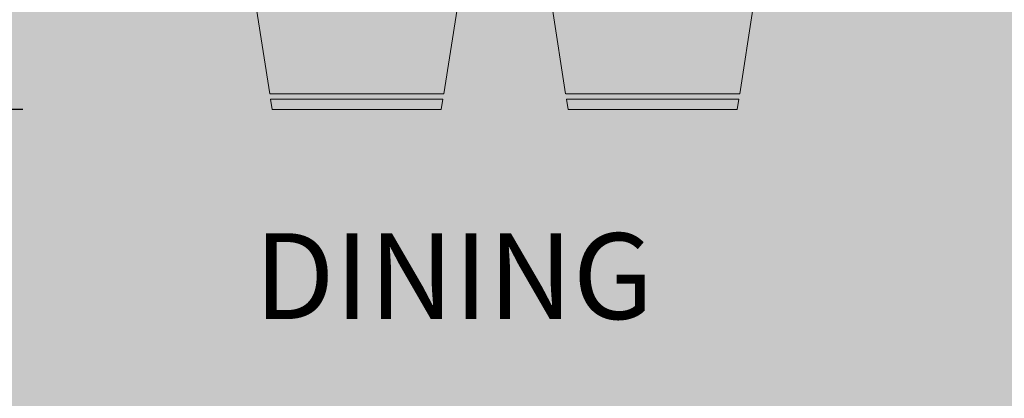
# Model space of a CAD drawing. Units: inches. Extents: x 3024 to 3952, y 1308 to 1863.
# Tile 7 of 29: x 3323 to 3392, y 1560 to 1587. Entities that reach past the tile are written whole.
import ezdxf

# ---------------------------------------------------------------- set-up
doc = ezdxf.new("R2010")
doc.units = ezdxf.units.IN
for name, color, linetype, lineweight in [('A-ANNO-DIMS', 2, 'Continuous', 18), ('A-AREA-IDEN', 7, 'Continuous', 18), ('A-FLOR-TILE-PATT', 7, 'Continuous', 13), ('A-FURN', 8, 'Continuous', 18), ('A-FURN-PATT', 9, 'Continuous', 13)]:
    doc.layers.add(name, color=color, linetype=linetype, lineweight=lineweight)
doc.layers.add('A-FLOR-PATT', color=254, linetype='Continuous', lineweight=13, true_color=0xfeeab9)
doc.styles.get("Standard").update_dxf_attribs({"font": 'arial.ttf'})
doc.dimstyles.get("Standard").update_dxf_attribs({"dimtxt": 0.18, "dimasz": 0.18, "dimexe": 0.18, "dimexo": 0.0625, "dimgap": 0.09, "dimtad": 0, "dimtih": 1, "dimtoh": 1, "dimdec": 4, "dimzin": 0, "dimdsep": 46, "dimtxsty": 'Standard', "dimcen": 0.09, "dimadec": 0, "dimazin": 0, "dimtfac": 1, "dimtdec": 4, "dimtofl": 0, "dimtmove": 0, "dimatfit": 3, "dimfxl": 1, "dimtolj": 1, "dimtzin": 0, "dimarcsym": 0})

# ---------------------------------------------------------------- blocks, each defined once
blk = doc.blocks.new('Dining Set - 36 x 72 in.')
for p, q in [((-22, 27.5), (-22.1562, 26.50042)), ((-22, 27.5), (-6, 27.5)), ((-5.8437, 26.49966), (-6, 27.5)), ((6, 27.5), (5.8438, 26.50042)), ((6, 27.5), (22, 27.5)), ((22.1563, 26.49966), (22, 27.5)), ((-5.8416, 26.5), (-22.1534, 26.5)), ((22.1584, 26.5), (5.8466, 26.5)), ((-22.2343, 26.00059), (-23.4847, 17.99762)), ((-22.2304, 26), (-5.7608, 26)), ((-4.5152, 17.99762), (-5.7655, 25.99926)), ((5.7657, 26.00059), (4.5153, 17.99762)), ((5.7696, 26), (22.2392, 26)), ((23.4848, 17.99762), (22.2345, 25.99926)), ((36, 18), (-36, 18)), ((-36, 18), (-36, -18)), ((36, -18), (36, 18)), ((-44.0006, 8.23428), (-35.9976, 9.48474)), ((44.0006, 8.23428), (35.9976, 9.48474)), ((-45.5, 8), (-44.5004, 8.15617)), ((-45.5, 8), (-45.5, -8)), ((-44.5, -8.15843), (-44.5, 8.15338)), ((-44, 8.23041), (-44, -8.23915)), ((44, 8.23041), (44, -8.23915)), ((44.5, -8.15843), (44.5, 8.15338)), ((45.5, 8), (44.5005, 8.15617)), ((45.5, 8), (45.5, -8)), ((-44.4997, -8.15631), (-45.5, -8)), ((-35.9976, -9.48476), (-43.9993, -8.2345)), ((35.9976, -9.48476), (43.9993, -8.2345)), ((44.4997, -8.15631), (45.5, -8)), ((-36, -18), (36, -18)), ((-22.2343, -26.0006), (-23.4847, -17.99762)), ((-4.5152, -17.99762), (-5.7655, -25.99928)), ((5.7657, -26.0006), (4.5153, -17.99762)), ((23.4848, -17.99762), (22.2345, -25.99928)), ((-22.2304, -26), (-5.7608, -26)), ((5.7696, -26), (22.2392, -26)), ((-22, -27.5), (-22.1562, -26.50044)), ((-5.8416, -26.5), (-22.1534, -26.5)), ((-5.8437, -26.49967), (-6, -27.5)), ((6, -27.5), (5.8438, -26.50044)), ((22.1584, -26.5), (5.8466, -26.5)), ((22.1563, -26.49967), (22, -27.5)), ((-22, -27.5), (-6, -27.5)), ((6, -27.5), (22, -27.5))]:
    blk.add_line(p, q)
for points in [[(-36, 15), (-31.1772, 14.97754), (-26.8079, 14.91406), (-22.8538, 14.81543), (-19.276, 14.6875), (-16.0362, 14.53613), (-13.0957, 14.36718), (-10.4159, 14.18652), (-7.9583, 14), (-5.6904, 13.81315), (-3.6035, 13.63021), (-1.6954, 13.45508), (0.0365, 13.29166), (1.5945, 13.14388), (2.9811, 13.01562), (4.1988, 12.9108), (5.25, 12.83333), (6.1393, 12.78613), (6.8802, 12.76823), (7.4883, 12.77767), (7.9792, 12.8125), (8.3685, 12.87077), (8.6719, 12.95052), (8.9049, 13.0498), (9.0833, 13.16666), (9.2205, 13.29899), (9.3216, 13.44401), (9.3895, 13.59879), (9.4271, 13.76041), (9.4373, 13.92594), (9.4232, 14.09245), (9.3875, 14.257), (9.3333, 14.41666), (9.2638, 14.56917), (9.1836, 14.71484), (9.0975, 14.85465), (9.0104, 14.98958), (8.9272, 15.1206), (8.8529, 15.2487), (8.7922, 15.37483), (8.75, 15.5), (8.7305, 15.62467), (8.7344, 15.74739), (8.7617, 15.86621), (8.8125, 15.97916), (8.8867, 16.08431), (8.9844, 16.17968), (9.1055, 16.26334), (9.25, 16.33333), (9.4189, 16.38802), (9.6172, 16.42708), (9.8506, 16.45052), (10.125, 16.45833), (10.4463, 16.45052), (10.8203, 16.42708), (11.2529, 16.38802), (11.75, 16.33333), (12.3184, 16.26318), (12.9694, 16.17838), (13.7151, 16.07991), (14.5677, 15.96875), (15.5395, 15.84586), (16.6426, 15.71224), (17.8893, 15.56884), (19.2917, 15.41666), (20.859, 15.25667), (22.5879, 15.08984), (24.4721, 14.91715), (26.5052, 14.73958), (28.6809, 14.5581), (30.9929, 14.3737), (33.4347, 14.18733), (36, 14)], [(-36, 10), (-28.9766, 10.14274), (-23.1725, 10.20442), (-18.4241, 10.19775), (-14.5677, 10.13541), (-11.4399, 10.03011), (-8.877, 9.89453), (-6.7154, 9.74137), (-4.7917, 9.58333), (-2.9698, 9.43082), (-1.2246, 9.28515), (0.4415, 9.14534), (2.026, 9.01041), (3.5266, 8.87939), (4.9408, 8.7513), (6.266, 8.62516), (7.5, 8.5), (8.6411, 8.37549), (9.6914, 8.2539), (10.6538, 8.13818), (11.5312, 8.03125), (12.3267, 7.93603), (13.043, 7.85547), (13.6831, 7.79248), (14.25, 7.75), (14.7471, 7.7303), (15.1797, 7.73307), (15.5537, 7.75732), (15.875, 7.80208), (16.1494, 7.86637), (16.3828, 7.94922), (16.5811, 8.04964), (16.75, 8.16666), (16.8944, 8.29915), (17.0143, 8.44531), (17.1089, 8.60319), (17.1771, 8.77083), (17.218, 8.94629), (17.2305, 9.1276), (17.2137, 9.31282), (17.1667, 9.5), (17.0895, 9.6875), (16.987, 9.875), (16.8649, 10.0625), (16.7292, 10.25), (16.5856, 10.4375), (16.4401, 10.625), (16.2985, 10.8125), (16.1667, 11), (16.05, 11.18733), (15.9518, 11.3737), (15.8752, 11.5581), (15.8229, 11.73958), (15.798, 11.91715), (15.8034, 12.08984), (15.842, 12.25667), (15.9167, 12.41666), (16.0295, 12.56836), (16.1784, 12.70833), (16.3605, 12.83268), (16.5729, 12.9375), (16.8127, 13.01888), (17.0768, 13.07291), (17.3625, 13.0957), (17.6667, 13.08333), (17.9894, 13.03312), (18.3418, 12.94726), (18.7382, 12.82918), (19.1927, 12.68229), (19.7195, 12.51001), (20.3327, 12.31575), (21.0465, 12.10294), (21.875, 11.875), (22.8357, 11.63354), (23.959, 11.37304), (25.2786, 11.08618), (26.8282, 10.76562), (28.6414, 10.40405), (30.752, 9.99414), (33.1936, 9.52856), (36, 9)], [(-36, 5.5), (-30.7157, 5.3348), (-26.069, 5.20963), (-21.9946, 5.11767), (-18.4271, 5.05208), (-15.3009, 5.00602), (-12.5508, 4.97265), (-10.1112, 4.94515), (-7.9167, 4.91666), (-5.909, 4.88167), (-4.0586, 4.83984), (-2.3429, 4.79215), (-0.7396, 4.73958), (0.7739, 4.6831), (2.22, 4.6237), (3.6213, 4.56233), (5, 4.5), (6.373, 4.43782), (7.7344, 4.3776), (9.0723, 4.32129), (10.375, 4.27083), (11.6309, 4.22819), (12.8281, 4.19531), (13.9551, 4.17415), (15, 4.16666), (15.954, 4.17448), (16.819, 4.19791), (17.6001, 4.23698), (18.3021, 4.29166), (18.9299, 4.36198), (19.4883, 4.44791), (19.9823, 4.54948), (20.4167, 4.66666), (20.7969, 4.79899), (21.1302, 4.94401), (21.4245, 5.09879), (21.6875, 5.26041), (21.9271, 5.42594), (22.1511, 5.59245), (22.3672, 5.757), (22.5834, 5.91666), (22.8065, 6.06868), (23.0404, 6.21093), (23.2879, 6.34147), (23.5521, 6.45833), (23.8358, 6.55957), (24.142, 6.64323), (24.4735, 6.70735), (24.8334, 6.75), (25.2235, 6.76969), (25.642, 6.76692), (26.0858, 6.74267), (26.5521, 6.69791), (27.0379, 6.63362), (27.5404, 6.55078), (28.0565, 6.45036), (28.5834, 6.33333), (29.1242, 6.19987), (29.7071, 6.04687), (30.3661, 5.87044), (31.1354, 5.66666), (32.0493, 5.43164), (33.142, 5.16146), (34.4475, 4.85221), (36, 4.5)], [(-36, -1), (-30.7915, -0.6591), (-26.0195, -0.38216), (-21.6519, -0.16284), (-17.6563, 0.00521), (-14.0005, 0.12833), (-10.6523, 0.21289), (-7.5796, 0.26522), (-4.75, 0.29166), (-2.134, 0.29793), (0.2878, 0.28711), (2.5317, 0.26163), (4.6146, 0.22396), (6.5529, 0.17651), (8.3633, 0.12174), (10.0623, 0.06209), (11.6667, 0), (13.1899, -0.06201), (14.6341, -0.1211), (15.9982, -0.17432), (17.2813, -0.21875), (18.4823, -0.25147), (19.6003, -0.26953), (20.6343, -0.27002), (21.5834, -0.25), (22.4481, -0.20768), (23.2357, -0.14584), (23.9549, -0.06836), (24.6146, 0.02083), (25.2235, 0.11784), (25.7904, 0.21875), (26.3241, 0.31966), (26.8334, 0.41666), (27.3265, 0.50618), (27.8099, 0.58593), (28.2894, 0.65397), (28.7709, 0.70833), (29.2601, 0.74707), (29.763, 0.76823), (30.2855, 0.76985), (30.8334, 0.75), (31.4088, 0.70784), (31.9994, 0.64713), (32.589, 0.57275), (33.1615, 0.48958), (33.7008, 0.4025), (34.1908, 0.3164), (34.6153, 0.23616), (34.9584, 0.16666), (35.2099, 0.11165), (35.3848, 0.07031), (35.504, 0.04069), (35.5886, 0.02083), (35.6594, 0.00879), (35.7377, 0.0026), (35.8442, 0.00032), (36, 0)], [(-36, -6.5), (-27.1843, -6.31267), (-20.084, -6.1263), (-14.469, -5.9419), (-10.1094, -5.76042), (-6.7752, -5.58285), (-4.2363, -5.41016), (-2.2629, -5.24333), (-0.625, -5.08334), (0.8708, -4.93099), (2.2715, -4.78646), (3.5872, -4.64974), (4.8281, -4.52084), (6.0046, -4.39974), (7.127, -4.28646), (8.2053, -4.18099), (9.25, -4.08334), (10.2705, -3.99382), (11.2734, -3.91407), (12.2647, -3.84603), (13.25, -3.79167), (14.2354, -3.75293), (15.2266, -3.73177), (16.2295, -3.73015), (17.25, -3.75), (18.2912, -3.79248), (19.3451, -3.85547), (20.4009, -3.93604), (21.4479, -4.03125), (22.4754, -4.13819), (23.4727, -4.25391), (24.4289, -4.37549), (25.3334, -4.5), (26.1785, -4.62492), (26.9694, -4.74935), (27.7145, -4.87281), (28.4219, -4.99479), (29.1, -5.11483), (29.7572, -5.23242), (30.4016, -5.34709), (31.0417, -5.45834), (31.6837, -5.56437), (32.3262, -5.65821), (32.9658, -5.73153), (33.599, -5.77604), (34.2224, -5.78345), (34.8327, -5.74545), (35.4264, -5.65373), (36, -5.5)], [(-36, -10), (-26.4022, -9.81299), (-18.4675, -9.62891), (-11.9839, -9.45069), (-6.7396, -9.28125), (-2.5226, -9.12354), (0.8789, -8.98047), (3.6769, -8.85498), (6.0833, -8.75), (8.2767, -8.66765), (10.3021, -8.60677), (12.1712, -8.56543), (13.8958, -8.54167), (15.4876, -8.53353), (16.9583, -8.53907), (18.3197, -8.55632), (19.5834, -8.58334), (20.7616, -8.61841), (21.8685, -8.66081), (22.9188, -8.71004), (23.9271, -8.76563), (24.9081, -8.82707), (25.8763, -8.89388), (26.8465, -8.96558), (27.8334, -9.04167), (28.8474, -9.12118), (29.8828, -9.20117), (30.93, -9.27824), (31.9792, -9.34896), (33.0205, -9.40991), (34.0443, -9.45768), (35.0407, -9.48885), (36, -9.5)], [(-36, -14.5), (-30.0881, -14.33513), (-25.0332, -14.21224), (-20.7312, -14.12647), (-17.0781, -14.07292), (-13.97, -14.04671), (-11.3027, -14.04297), (-8.9724, -14.05681), (-6.875, -14.08334), (-4.9224, -14.11833), (-3.0905, -14.16016), (-1.3709, -14.20785), (0.2448, -14.26042), (1.7647, -14.3169), (3.1973, -14.3763), (4.5507, -14.43767), (5.8333, -14.5), (7.0554, -14.5621), (8.235, -14.62175), (9.3922, -14.67652), (10.5469, -14.72396), (11.7192, -14.76164), (12.929, -14.78711), (14.1965, -14.79794), (15.5417, -14.79167), (16.9933, -14.76424), (18.6152, -14.70508), (20.4804, -14.60197), (22.6615, -14.44271), (25.2312, -14.21509), (28.2624, -13.9069), (31.8277, -13.50594), (36, -13)]]:
    blk.add_lwpolyline(points)
blk = doc.blocks.new('*D21')
at = {"layer": 'A-ANNO-DIMS', "color": 0, "lineweight": -2, "transparency": 16777216}
for p, q in [((3323.055, 1621.114), (3312.873, 1621.114)), ((3313.053, 1620.934), (3313.053, 1601.018)), ((3313.053, 1580.742), (3313.053, 1600.657)), ((3323.055, 1580.562), (3312.873, 1580.562))]:
    blk.add_line(p, q, dxfattribs=at)
at = {"layer": 'A-ANNO-DIMS', "color": 0, "transparency": 16777216}
for points in [[(3313.023, 1620.934), (3313.083, 1620.934), (3313.053, 1621.114)], [(3313.023, 1580.742), (3313.083, 1580.742), (3313.053, 1580.562)]]:
    blk.add_solid(points, dxfattribs=at)
at = {"layer": 'Defpoints', "color": 0, "transparency": 16777216}
for p in [(3313.053, 1621.114), (3323.117, 1621.114), (3323.117, 1580.562)]:
    blk.add_point(p, dxfattribs=at)
at = {"layer": 'A-ANNO-DIMS', "color": 0, "transparency": 16777216, "insert": (3313.053, 1600.838), "char_height": 0.18, "attachment_point": 5}
blk.add_mtext('\\A1;41', dxfattribs=at)

msp = doc.modelspace()

# ---------------------------------------------------------------- hatches: boundary and pattern name
at = {"layer": 'A-FLOR-PATT', "transparency": 33554528}
h = msp.add_hatch(color=256, dxfattribs=at)
h.dxf.hatch_style = 1
h.paths.add_polyline_path([(3460.764, 1688.6064), (3412.764, 1688.6064), (3412.764, 1694.6064), (3460.764, 1694.6064), (3460.764, 1778.6064), (3406.764, 1778.6064), (3406.764, 1759.9514), (3318.2981, 1759.9514), (3318.2981, 1658.6064), (3322.5356, 1658.6064), (3322.5356, 1652.6064), (3292.764, 1652.6064), (3292.764, 1778.6064), (3106.764, 1778.6064), (3106.764, 1628.6064), (3172.764, 1628.6064), (3172.764, 1532.6064), (3166.764, 1532.6064), (3166.764, 1628.6064), (3106.764, 1628.6064), (3106.764, 1356.8452), (3202.812, 1356.8452), (3202.812, 1354.2534), (3202.812, 1353.8388), (3202.812, 1351.1212), (3202.812, 1347.8452), (3277.764, 1347.8452), (3277.764, 1353.8452), (3277.764, 1356.8452), (3277.764, 1442.6064), (3460.764, 1442.6064)])
h.paths.add_polyline_path([(3216.238, 1527.2064), (3216.238, 1491.2064), (3214.663, 1491.2064), (3214.663, 1491.2409, -0.3966224), (3180.243, 1526.6064), (3163.0285, 1526.6064), (3163.0285, 1531.1064), (3161.716, 1531.1064), (3161.716, 1561.1064), (3163.0285, 1561.1064), (3163.0285, 1531.1064), (3163.0285, 1526.6064), (3180.243, 1526.6064, 0.3966224), (3214.663, 1491.2409), (3214.663, 1527.2064)], flags=16)
h.paths.add_polyline_path([(3227.364, 1649.8972), (3191.364, 1649.8972), (3191.364, 1651.4722), (3227.364, 1651.4722)], flags=16)
h.paths.add_polyline_path([(3323.1172, 1606.7362), (3323.8545, 1606.8514), (3323.8545, 1594.8241), (3323.1172, 1594.9393)], flags=16)
h.paths.add_polyline_path([(3324.2232, 1606.909), (3330.1216, 1607.8307), (3330.1216, 1614.1093), (3339.3495, 1614.1093), (3340.2711, 1620.0078), (3352.4136, 1620.0078), (3353.3353, 1614.1093), (3359.9941, 1614.1093), (3360.9157, 1620.0078), (3373.0582, 1620.0078), (3373.9799, 1614.1093), (3383.2077, 1614.1093), (3383.2077, 1607.8307), (3389.1062, 1606.909), (3389.1062, 1594.7665), (3383.2077, 1593.8449), (3383.2077, 1587.5663), (3373.9799, 1587.5663), (3373.0583, 1581.6678), (3360.9157, 1581.6678), (3359.9941, 1587.5663), (3353.3353, 1587.5663), (3352.4136, 1581.6678), (3340.2711, 1581.6678), (3339.3495, 1587.5663), (3330.1216, 1587.5663), (3330.1216, 1593.8449), (3324.2232, 1594.7665)], flags=16)
h.paths.add_polyline_path([(3236.1584, 1693.1064), (3236.1584, 1723.1064), (3237.4709, 1723.1064), (3237.4709, 1693.1064)], flags=16)
h.paths.add_polyline_path([(3373.2158, 1600.6847), (3373.7965, 1600.7303), (3374.3268, 1600.7874), (3374.8132, 1600.8531), (3375.2621, 1600.9247), (3375.6801, 1600.9991), (3376.0736, 1601.0735), (3376.6855, 1601.19), (3377.366, 1601.3023), (3378.0667, 1601.3814), (3378.8026, 1601.4123), (3379.5865, 1601.3839), (3380.4537, 1601.2948), (3381.301, 1601.1717), (3382.0317, 1601.0433), (3382.4398, 1600.9607), (3382.6252, 1600.9201), (3382.919, 1600.8507), (3382.9044, 1600.8531), (3382.842, 1600.8678), (3382.7541, 1600.8896), (3382.6252, 1600.9201), (3382.4398, 1600.9607), (3382.1868, 1601.0119), (3381.8738, 1601.0711), (3381.5125, 1601.1346), (3381.1149, 1601.1988), (3380.6928, 1601.2601), (3380.2581, 1601.3149), (3379.8226, 1601.3597), (3379.3984, 1601.3908), (3378.9944, 1601.4054), (3378.6092, 1601.4042), (3378.2384, 1601.3886), (3377.8777, 1601.36), (3377.5227, 1601.32), (3377.1691, 1601.2698), (3376.8127, 1601.211), (3376.4491, 1601.145), (3376.0736, 1601.0735), (3375.4177, 1600.9494), (3374.5542, 1600.8119), (3373.5044, 1600.6988)], flags=0)
h.paths.add_polyline_path([(3380.0253, 1596.7351), (3380.499, 1596.6659), (3380.9706, 1596.6119), (3381.4375, 1596.5791), (3381.8971, 1596.5736), (3382.5886, 1596.6167), (3382.7848, 1596.6692), (3382.1465, 1596.5706), (3381.236, 1596.5815), (3380.3199, 1596.6865)], flags=0)
h.paths.add_polyline_path([(3369.6414, 1603.9617), (3370.1589, 1604.0021), (3370.6218, 1604.0539), (3371.0335, 1604.1173), (3371.3978, 1604.1921), (3371.7181, 1604.2785), (3371.9984, 1604.3761), (3372.2441, 1604.483), (3372.4611, 1604.5972), (3372.655, 1604.7163), (3372.8317, 1604.8384), (3372.9968, 1604.9611), (3373.3703, 1605.2455), (3373.8426, 1605.5328), (3374.4624, 1605.7539), (3375.1058, 1605.8302), (3375.7221, 1605.8261), (3376.4109, 1605.76), (3377.1534, 1605.6376), (3377.8945, 1605.473), (3378.1382, 1605.409), (3377.7394, 1605.5074), (3377.3509, 1605.5937), (3376.9704, 1605.6677), (3376.5999, 1605.7288), (3376.2417, 1605.7762), (3375.8979, 1605.8092), (3375.5707, 1605.8271), (3375.2621, 1605.8291), (3374.9745, 1605.8146), (3374.7092, 1605.7832), (3374.4647, 1605.7359), (3374.239, 1605.6742), (3374.0298, 1605.5996), (3373.835, 1605.5134), (3373.6525, 1605.4171), (3373.4801, 1605.3123), (3373.3156, 1605.2002), (3373.1562, 1605.0825), (3372.7603, 1604.781), (3372.236, 1604.4588), (3371.5738, 1604.2283), (3370.8493, 1604.0794), (3369.9262, 1603.976)], flags=0)
h.paths.add_polyline_path([(3366.7533, 1606.5832), (3367.1713, 1606.5519), (3367.5378, 1606.5374), (3367.8568, 1606.5394), (3368.1325, 1606.5573), (3368.3694, 1606.5903), (3368.5717, 1606.6377), (3368.7438, 1606.6988), (3368.89, 1606.7728), (3369.0146, 1606.8591), (3369.121, 1606.9568), (3369.2094, 1607.0646), (3369.2792, 1607.181), (3369.3295, 1607.3046), (3369.3596, 1607.4339), (3369.3688, 1607.5676), (3369.3565, 1607.7042), (3369.3218, 1607.8422), (3369.2649, 1607.9804), (3369.1893, 1608.1187), (3369.0993, 1608.2569), (3368.9992, 1608.3952), (3368.8934, 1608.5334), (3368.7861, 1608.6717), (3368.6817, 1608.8099), (3368.4212, 1609.1804), (3368.2685, 1609.7106), (3368.4883, 1610.1814), (3369.0537, 1610.4604), (3369.6717, 1610.5097), (3370.2812, 1610.3612), (3370.4805, 1610.2968), (3370.1882, 1610.3839), (3369.9284, 1610.4472), (3369.6905, 1610.4842), (3369.4662, 1610.4933), (3369.2555, 1610.4765), (3369.0608, 1610.4367), (3368.884, 1610.3767), (3368.7274, 1610.2994), (3368.5931, 1610.2077), (3368.4833, 1610.1045), (3368.4002, 1609.9927), (3368.3451, 1609.8747), (3368.3166, 1609.7517), (3368.3127, 1609.6244), (3368.331, 1609.4935), (3368.3696, 1609.3597), (3368.4261, 1609.2237), (3368.4985, 1609.0863), (3368.5845, 1608.9482), (3368.6817, 1608.8099), (3368.7861, 1608.6717), (3368.8934, 1608.5334), (3368.9992, 1608.3952), (3369.0993, 1608.2569), (3369.3398, 1607.8876), (3369.3941, 1607.2896), (3368.9774, 1606.7817), (3368.3928, 1606.5742), (3367.7162, 1606.5303), (3367.0044, 1606.5585)], flags=0)
h.paths.add_polyline_path([(3362.1859, 1610.2589), (3362.5478, 1610.2845), (3362.8348, 1610.3275), (3363.0585, 1610.3863), (3363.2303, 1610.4595), (3363.3619, 1610.5457), (3363.463, 1610.6432), (3363.5376, 1610.7502), (3363.5876, 1610.8643), (3363.6153, 1610.9834), (3363.6229, 1611.1055), (3363.6125, 1611.2283), (3363.5861, 1611.3496), (3363.5462, 1611.4673), (3363.4949, 1611.5797), (3363.4358, 1611.6871), (3363.3723, 1611.7902), (3363.3081, 1611.8897), (3363.2468, 1611.9863), (3363.192, 1612.0808), (3363.0258, 1612.4261), (3363.3371, 1612.8672), (3363.9008, 1612.9782), (3364.4822, 1612.9641), (3365.1098, 1612.9074), (3365.328, 1612.8805), (3364.9615, 1612.9208), (3364.6426, 1612.9496), (3364.3668, 1612.9669), (3364.1299, 1612.9726), (3363.9276, 1612.9669), (3363.7555, 1612.9496), (3363.6093, 1612.9208), (3363.4848, 1612.8805), (3363.3782, 1612.8289), (3363.2889, 1612.7672), (3363.2169, 1612.6969), (3363.1622, 1612.6193), (3363.1247, 1612.5361), (3363.1046, 1612.4484), (3363.1017, 1612.358), (3363.1161, 1612.266), (3363.1472, 1612.1738), (3363.192, 1612.0808), (3363.2468, 1611.9863), (3363.3081, 1611.8897), (3363.3723, 1611.7902), (3363.4358, 1611.6871), (3363.6363, 1611.323), (3363.5979, 1610.7003), (3363.0863, 1610.3651), (3362.3983, 1610.2622)], flags=0)
h.paths.add_polyline_path([(3352.356, 1581.2991), (3352.2408, 1580.5618), (3340.4439, 1580.5618), (3340.3287, 1581.2991)], flags=16)
h.paths.add_polyline_path([(3340.4439, 1621.1137), (3352.2408, 1621.1137), (3352.356, 1620.3764), (3340.3287, 1620.3764)], flags=16)
h.paths.add_polyline_path([(3278.4282, 1504.7424), (3290.3831, 1504.7424), (3290.3831, 1502.7499), (3291.0473, 1502.7499), (3291.0473, 1494.7799), (3290.3831, 1494.7799), (3290.3831, 1494.1158), (3291.0473, 1494.1158), (3291.0473, 1486.1458), (3290.3831, 1486.1458), (3290.3831, 1484.1533), (3291.0473, 1484.1533), (3291.0473, 1483.4892, -0.0909091), (3291.0473, 1468.8776), (3291.0473, 1468.2135), (3290.3831, 1468.2135), (3290.3831, 1464.8926), (3278.4282, 1464.8926), (3278.4282, 1472.8626), (3277.764, 1473.5268), (3277.764, 1478.84), (3278.4282, 1479.5042)], flags=16)
h.paths.add_polyline_path([(3278.7603, 1504.4103), (3290.051, 1504.4103), (3290.051, 1465.2247), (3278.7603, 1465.2247)], flags=0)
h.paths.add_polyline_path([(3123.904, 1600.7821), (3117.9039, 1602.7821), (3117.9039, 1599.7821), (3119.4039, 1599.7821), (3119.4039, 1596.7821), (3118.4039, 1596.7821), (3118.4039, 1598.7821), (3117.9039, 1598.7821), (3117.9039, 1596.2821), (3109.9039, 1596.2821), (3109.9039, 1617.2821), (3117.9039, 1617.2821), (3117.9039, 1610.7821), (3123.9038, 1612.7821, -0.7025712), (3137.9039, 1606.7822, -0.7025621)], flags=16)
h.paths.add_polyline_path([(3123.9039, 1602.7822), (3123.9039, 1610.7822, -0.7345333), (3136.9039, 1606.7822, -0.7345297)], flags=0)
h.paths.add_polyline_path([(3177.972, 1689.6473), (3109.2405, 1689.6473), (3109.2405, 1741.1959), (3177.972, 1741.1959)], flags=16)
h.paths.add_polyline_path([(3373.0006, 1581.2991), (3372.8854, 1580.5618), (3361.0885, 1580.5618), (3360.9733, 1581.2991)], flags=16)
h.paths.add_polyline_path([(3361.0885, 1621.1137), (3372.8854, 1621.1137), (3373.0006, 1620.3764), (3360.9733, 1620.3764)], flags=16)
h.paths.add_polyline_path([(3116.9039, 1598.2821, -0.4142136), (3116.1539, 1597.2821), (3111.9039, 1597.2821, -0.4142136), (3110.9039, 1598.0321), (3110.9039, 1615.2821, -0.4142136), (3111.6539, 1616.2821), (3115.9039, 1616.2821, -0.4142136), (3116.9039, 1615.5321)], flags=0)
h.paths.add_polyline_path([(3121.6122, 1728.1369), (3121.6122, 1696.5205), (3110.2715, 1696.5205), (3110.2715, 1714.3906), (3121.6122, 1714.3906), (3121.6122, 1716.4526), (3110.2715, 1716.4526), (3110.2715, 1734.3228), (3123.3304, 1734.3228), (3123.3304, 1729.8552), (3134.6711, 1741.1959), (3134.6711, 1728.1369)], flags=0)
h.paths.add_polyline_path([(3389.4748, 1606.8514), (3390.2122, 1606.7362), (3390.2122, 1594.9393), (3389.4748, 1594.8241)], flags=16)
h.paths.add_polyline_path([(3257.6842, 1762.8281), (3259.6842, 1768.8281), (3256.6842, 1768.8281), (3256.6842, 1767.3281), (3253.6842, 1767.3281), (3253.6842, 1768.3281), (3255.6842, 1768.3281), (3255.6842, 1768.8281), (3253.1842, 1768.8281), (3253.1842, 1776.8281), (3274.1842, 1776.8281), (3274.1842, 1768.8281), (3267.6842, 1768.8281), (3269.6842, 1762.8282, -0.7025712), (3263.6843, 1748.8282, -0.7025621)], flags=16)
h.paths.add_polyline_path([(3259.6842, 1762.8281), (3267.6843, 1762.8281, -0.7345333), (3263.6842, 1749.8282, -0.7345297)], flags=0)
h.paths.add_polyline_path([(3411.264, 1715.6064), (3411.264, 1716.9189), (3441.264, 1716.9189), (3441.264, 1715.6064)], flags=16)
h.paths.add_polyline_path([(3178.3806, 1449.1876), (3178.3806, 1397.639), (3109.6491, 1397.639), (3109.6491, 1449.1876)], flags=16)
h.paths.add_polyline_path([(3397.1501, 1541.7146), (3419.6183, 1541.7146), (3419.6183, 1496.7783), (3397.1501, 1496.7783)], flags=16)
h.paths.add_polyline_path([(3254.1842, 1770.5781), (3254.1842, 1774.8281, -0.4142136), (3254.9342, 1775.8281), (3272.1842, 1775.8281, -0.4142136), (3273.1842, 1775.0781), (3273.1842, 1770.8281, -0.4142136), (3272.4342, 1769.8281), (3255.1842, 1769.8281, -0.4142136)], flags=0)
h.paths.add_polyline_path([(3403.672, 1500.7601), (3403.6016, 1500.3997), (3403.5328, 1500.0441), (3403.4662, 1499.6867), (3403.4027, 1499.3226), (3403.3464, 1498.9532), (3403.3025, 1498.5811), (3403.2759, 1498.2091), (3403.2714, 1497.8401), (3403.3064, 1497.2813), (3403.3491, 1497.1219), (3403.2689, 1497.6395), (3403.2778, 1498.3719), (3403.3635, 1499.0984), (3403.4889, 1499.8168), (3403.6016, 1500.3997), (3403.672, 1500.7601), (3403.744, 1501.1315), (3403.817, 1501.5205), (3403.891, 1501.9336), (3403.9656, 1502.3769), (3404.0404, 1502.8572), (3404.115, 1503.3786), (3404.2264, 1504.2311), (3404.2571, 1504.5223), (3404.1552, 1503.6598), (3404.0063, 1502.6193), (3403.8604, 1501.7518), (3403.744, 1501.1315)], flags=0)
h.paths.add_polyline_path([(3406.5868, 1505.0416), (3406.6121, 1504.5236), (3406.6492, 1504.0526), (3406.6956, 1503.624), (3406.7491, 1503.2333), (3406.8072, 1502.8759), (3406.8676, 1502.5473), (3406.9281, 1502.243), (3407.0268, 1501.7597), (3407.1416, 1501.1368), (3407.2087, 1500.3904), (3407.1804, 1499.6703), (3407.1078, 1498.9956), (3407.0074, 1498.3199), (3406.8809, 1497.6059), (3406.7403, 1496.9627), (3406.7418, 1496.9824), (3406.7491, 1497.0249), (3406.8229, 1497.3409), (3406.8364, 1497.4025), (3406.878, 1497.6078), (3406.9261, 1497.8614), (3406.9777, 1498.1526), (3407.0298, 1498.4712), (3407.0797, 1498.8068), (3407.1243, 1499.149), (3407.1607, 1499.4874), (3407.1859, 1499.8115), (3407.1978, 1500.1137), (3407.1969, 1500.3962), (3407.1841, 1500.6642), (3407.1609, 1500.9225), (3407.1284, 1501.1761), (3407.0876, 1501.43), (3407.0398, 1501.6891), (3406.9862, 1501.9585), (3406.8832, 1502.4628), (3406.7712, 1503.0713), (3406.6657, 1503.8424), (3406.5924, 1504.7735)], flags=0)
h.paths.add_polyline_path([(3409.2517, 1507.8962), (3409.2752, 1507.4282), (3409.3079, 1507.0076), (3409.3501, 1506.6314), (3409.4015, 1506.2969), (3409.4624, 1506.0009), (3409.5326, 1505.7406), (3409.6119, 1505.5128), (3409.6988, 1505.3131), (3409.7915, 1505.1368), (3409.8883, 1504.9792), (3409.9875, 1504.8356), (3410.0872, 1504.7015), (3410.1859, 1504.572), (3410.4508, 1504.2132), (3410.7205, 1503.6035), (3410.8059, 1502.8824), (3410.7619, 1502.0875), (3410.6122, 1501.2299), (3410.4402, 1500.6169), (3410.2538, 1500.0031), (3410.0536, 1499.3219), (3409.9909, 1499.0812), (3410.1761, 1499.7472), (3410.3596, 1500.3513), (3410.4512, 1500.6561), (3410.5312, 1500.9412), (3410.6013, 1501.226), (3410.6614, 1501.512), (3410.7111, 1501.7964), (3410.7496, 1502.0763), (3410.7764, 1502.3489), (3410.7909, 1502.6114), (3410.7926, 1502.8608), (3410.7808, 1503.0944), (3410.7553, 1503.31), (3410.7169, 1503.5087), (3410.6667, 1503.6921), (3410.6061, 1503.8621), (3410.5361, 1504.0203), (3410.4578, 1504.1686), (3410.3726, 1504.3088), (3410.2815, 1504.4424), (3410.1859, 1504.572), (3410.0872, 1504.7015), (3409.859, 1505.0083), (3409.5943, 1505.5117), (3409.4266, 1506.1336), (3409.324, 1506.8011), (3409.2586, 1507.6407)], flags=0)
h.paths.add_polyline_path([(3411.4914, 1510.5878), (3411.4432, 1510.1586), (3411.4054, 1509.775), (3411.38, 1509.4354), (3411.3681, 1509.1376), (3411.3698, 1508.8784), (3411.3843, 1508.6542), (3411.4112, 1508.4618), (3411.4497, 1508.2974), (3411.4994, 1508.1575), (3411.5595, 1508.0388), (3411.6296, 1507.9375), (3411.7097, 1507.851), (3411.802, 1507.7792), (3411.9096, 1507.7225), (3412.0353, 1507.6817), (3412.1821, 1507.6572), (3412.3528, 1507.6496), (3412.5505, 1507.6597), (3412.778, 1507.6879), (3413.0364, 1507.7341), (3413.3194, 1507.7955), (3413.6188, 1507.8687), (3413.9264, 1507.95), (3414.234, 1508.036), (3414.5333, 1508.1232), (3414.8163, 1508.208), (3415.0747, 1508.287), (3415.3023, 1508.3569), (3415.5007, 1508.4158), (3415.6733, 1508.4617), (3416.1158, 1508.5538), (3416.512, 1508.2591), (3416.716, 1507.6581), (3416.61, 1507.0003), (3416.3052, 1506.3411), (3415.8928, 1505.618), (3415.7339, 1505.3633), (3415.9914, 1505.791), (3416.201, 1506.1583), (3416.3666, 1506.4739), (3416.4925, 1506.7462), (3416.5828, 1506.9838), (3416.6413, 1507.1949), (3416.6725, 1507.3883), (3416.6799, 1507.5705), (3416.6662, 1507.7417), (3416.6339, 1507.9), (3416.5851, 1508.0436), (3416.5223, 1508.1709), (3416.4478, 1508.28), (3416.3639, 1508.3692), (3416.273, 1508.4368), (3416.1765, 1508.4815), (3416.0718, 1508.5047), (3415.9553, 1508.5079), (3415.8237, 1508.493), (3415.6733, 1508.4617), (3415.5007, 1508.4158), (3415.3327, 1508.3659), (3414.6495, 1508.157), (3414.0606, 1507.9855), (3413.4456, 1507.8229), (3412.8838, 1507.701), (3412.5505, 1507.6597), (3412.0748, 1507.6354), (3411.595, 1507.8883), (3411.398, 1508.4429), (3411.3624, 1508.9927), (3411.3854, 1509.5711), (3411.4578, 1510.3071)], flags=0)
h.paths.add_polyline_path([(3135.0797, 1449.1876), (3135.0797, 1436.1286), (3122.0208, 1436.1286), (3122.0208, 1404.5122), (3110.6801, 1404.5122), (3110.6801, 1422.3823), (3122.0208, 1422.3823), (3122.0208, 1424.4443), (3110.6801, 1424.4443), (3110.6801, 1442.3145), (3123.739, 1442.3145), (3123.739, 1437.8469)], flags=0)
h.paths.add_polyline_path([(3416.4944, 1514.2949), (3416.4837, 1513.8511), (3416.4893, 1513.4867), (3416.5102, 1513.1926), (3416.5451, 1512.9593), (3416.5929, 1512.7775), (3416.6524, 1512.6379), (3416.7224, 1512.531), (3416.8017, 1512.4488), (3416.8886, 1512.3882), (3416.9813, 1512.3476), (3417.0781, 1512.3251), (3417.1773, 1512.3189), (3417.277, 1512.3274), (3417.3757, 1512.3488), (3417.4713, 1512.3813), (3417.5627, 1512.4229), (3417.65, 1512.471), (3417.7338, 1512.5225), (3417.8146, 1512.5747), (3417.8931, 1512.6245), (3417.9699, 1512.6691), (3418.2968, 1512.8265), (3418.6505, 1512.4645), (3418.7037, 1511.9342), (3418.6693, 1511.3839), (3418.6076, 1510.8228), (3418.5777, 1510.5927), (3418.6197, 1510.9333), (3418.6525, 1511.2311), (3418.6759, 1511.4903), (3418.6899, 1511.7144), (3418.6946, 1511.9069), (3418.6899, 1512.0713), (3418.6759, 1512.2112), (3418.6525, 1512.33), (3418.6197, 1512.4311), (3418.5778, 1512.5177), (3418.5276, 1512.5903), (3418.4705, 1512.6488), (3418.4075, 1512.6933), (3418.3399, 1512.7237), (3418.2686, 1512.7401), (3418.1951, 1512.7424), (3418.1204, 1512.7307), (3418.0455, 1512.7055), (3417.9792, 1512.6736), (3417.65, 1512.471), (3417.5627, 1512.4229), (3417.4713, 1512.3813), (3417.3757, 1512.3488), (3417.277, 1512.3274), (3416.878, 1512.2936), (3416.5757, 1512.7549), (3416.492, 1513.3145), (3416.4808, 1514.0384)], flags=0)
h.paths.add_polyline_path([(3392.8223, 1481.9454), (3396.7707, 1481.9454), (3396.7707, 1480.9201), (3428.3585, 1480.9201), (3428.3585, 1481.9454), (3432.3069, 1481.9454), (3432.3069, 1464.8354, -0.266667), (3392.8223, 1464.8354)], flags=16)
h.paths.add_polyline_path([(3431.203, 1547.5428), (3450.8613, 1547.5428, -0.1904762), (3450.8614, 1484.031), (3431.203, 1484.031), (3431.203, 1488.5675), (3432.3809, 1488.5675), (3432.3809, 1543.0062), (3431.203, 1543.0062)], flags=16)
h.paths.add_polyline_path([(3451.9233, 1524.86, -0.0496282), (3451.9233, 1506.7138), (3446.7921, 1506.7138), (3446.7921, 1524.86)], flags=0)
h.paths.add_polyline_path([(3460.764, 1436.6064), (3277.764, 1436.6064), (3277.764, 1356.8452), (3277.764, 1353.8452), (3460.764, 1353.8452)], flags=17)
h.paths.add_polyline_path([(3121.3033, 1577.378), (3153.693, 1577.378), (3153.693, 1586.6752), (3121.3033, 1586.6752)], flags=24)
h.paths.add_polyline_path([(3164.1457, 1464.1276), (3210.4801, 1464.1276), (3210.4801, 1473.4247), (3164.1457, 1473.4247)], flags=24)
h.paths.add_polyline_path([(3343.1909, 1505.8863), (3373.7236, 1505.8863), (3373.7236, 1515.1773), (3343.1909, 1515.1773)], flags=24)
h.paths.add_polyline_path([(3337.6353, 1564.2926), (3370.0189, 1564.2926), (3370.0189, 1573.5836), (3337.6353, 1573.5836)], flags=24)
h.paths.add_polyline_path([(3419.204, 1753.8578), (3453.3997, 1753.8578), (3453.3997, 1762.9956), (3419.204, 1762.9956)], flags=24)
h.paths.add_polyline_path([(3341.2523, 1701.0246), (3381.0761, 1701.0246), (3381.0761, 1710.3156), (3341.2523, 1710.3156)], flags=24)
h.paths.add_polyline_path([(3245.8895, 1726.2997), (3278.2793, 1726.2997), (3278.2793, 1735.5968), (3245.8895, 1735.5968)], flags=24)
h.paths.add_polyline_path([(3128.8045, 1668.6736), (3175.1389, 1668.6736), (3175.1389, 1677.9707), (3128.8045, 1677.9707)], flags=24)
h.paths.add_polyline_path([(3345.9997, 1396.0062), (3389.09, 1396.0062), (3389.09, 1405.3033), (3345.9997, 1405.3033)], flags=24)
at = {"layer": 'A-FLOR-TILE-PATT', "transparency": 33554569}
h = msp.add_hatch(dxfattribs=at)
h.set_pattern_fill('ANGLE', color=256, scale=2)
h.set_pattern_definition([(0, (0, 0), (0, 13.97), [10.16, -3.81]), (90, (0, 0), (-13.97, 9e-16), [10.16, -3.81])])
h.paths.add_polyline_path([(3292.764, 1778.6064), (3232.764, 1778.6064), (3232.764, 1694.6064), (3236.1584, 1694.6064), (3236.1584, 1723.1064), (3237.4709, 1723.1064), (3237.4709, 1723.0777, -0.3870039), (3266.1209, 1694.6064), (3292.764, 1694.6064)])
h.paths.add_polyline_path([(3263.6843, 1748.8282, -0.7025621), (3257.6842, 1762.8281), (3259.6842, 1768.8281), (3256.6842, 1768.8281), (3256.6842, 1767.3281), (3253.6842, 1767.3281), (3253.6842, 1768.3281), (3255.6842, 1768.3281), (3255.6842, 1768.8281), (3253.1842, 1768.8281), (3253.1842, 1776.8281), (3274.1842, 1776.8281), (3274.1842, 1768.8281), (3267.6842, 1768.8281), (3269.6842, 1762.8282, -0.7025712)], flags=16)
h.paths.add_polyline_path([(3263.6842, 1749.8282, -0.7345297), (3259.6842, 1762.8281), (3267.6843, 1762.8281, -0.7345333)], flags=0)
h.paths.add_polyline_path([(3255.1842, 1769.8281, -0.4142136), (3254.1842, 1770.5781), (3254.1842, 1774.8281, -0.4142136), (3254.9342, 1775.8281), (3272.1842, 1775.8281, -0.4142136), (3273.1842, 1775.0781), (3273.1842, 1770.8281, -0.4142136), (3272.4342, 1769.8281)], flags=0)
h.paths.add_polyline_path([(3460.764, 1436.6064), (3277.764, 1436.6064), (3277.764, 1356.8452), (3277.764, 1353.8452), (3460.764, 1353.8452)])
h.paths.add_polyline_path([(3166.764, 1628.6064), (3106.764, 1628.6064), (3106.764, 1532.6064), (3133.066, 1532.6064, -0.3870039), (3161.716, 1561.0777), (3161.716, 1561.1064), (3163.0285, 1561.1064), (3163.0285, 1532.6064), (3166.764, 1532.6064)])
h.paths.add_polyline_path([(3123.904, 1600.7821), (3117.9039, 1602.7821), (3117.9039, 1599.7821), (3119.4039, 1599.7821), (3119.4039, 1596.7821), (3118.4039, 1596.7821), (3118.4039, 1598.7821), (3117.9039, 1598.7821), (3117.9039, 1596.2821), (3109.9039, 1596.2821), (3109.9039, 1617.2821), (3117.9039, 1617.2821), (3117.9039, 1610.7821), (3123.9038, 1612.7821, -0.7025712), (3137.9039, 1606.7822, -0.7025621)], flags=16)
h.paths.add_polyline_path([(3123.9039, 1602.7822), (3123.9039, 1610.7822, -0.7345333), (3136.9039, 1606.7822, -0.7345297)], flags=0)
h.paths.add_polyline_path([(3116.1539, 1597.2821), (3111.9039, 1597.2821, -0.4142136), (3110.9039, 1598.0321), (3110.9039, 1615.2821, -0.4142136), (3111.6539, 1616.2821), (3115.9039, 1616.2821, -0.4142136), (3116.9039, 1615.5321), (3116.9039, 1598.2821, -0.4142136)], flags=0)
h.paths.add_polyline_path([(3245.8895, 1726.2997), (3278.2793, 1726.2997), (3278.2793, 1735.5968), (3245.8895, 1735.5968)], flags=24)
h.paths.add_polyline_path([(3345.9997, 1396.0062), (3389.09, 1396.0062), (3389.09, 1405.3033), (3345.9997, 1405.3033)], flags=24)
h.paths.add_polyline_path([(3121.3033, 1577.378), (3153.693, 1577.378), (3153.693, 1586.6752), (3121.3033, 1586.6752)], flags=24)
at = {"layer": 'A-FURN-PATT', "transparency": 33554511}
h = msp.add_hatch(color=256, dxfattribs=at)
h.dxf.hatch_style = 1
h.paths.add_polyline_path([(3373.0582, 1620.0078), (3360.9157, 1620.0078), (3359.9941, 1614.1093), (3373.9799, 1614.1093)])
h.paths.add_polyline_path([(3372.8854, 1621.1137), (3361.0885, 1621.1137), (3360.9733, 1620.3764), (3373.0006, 1620.3764)])
h.paths.add_polyline_path([(3389.1062, 1606.909), (3383.2077, 1607.8307), (3383.2077, 1593.8449), (3389.1062, 1594.7665)])
h.paths.add_polyline_path([(3390.2122, 1606.7362), (3389.4748, 1606.8514), (3389.4748, 1594.8241), (3390.2122, 1594.9393)])
h.paths.add_polyline_path([(3373.9799, 1587.5663), (3359.9941, 1587.5663), (3360.9157, 1581.6678), (3373.0583, 1581.6678)])
h.paths.add_polyline_path([(3373.0006, 1581.2991), (3360.9733, 1581.2991), (3361.0885, 1580.5618), (3372.8854, 1580.5618)])
h.paths.add_polyline_path([(3353.3353, 1587.5663), (3339.3495, 1587.5663), (3340.2711, 1581.6678), (3352.4136, 1581.6678)])
h.paths.add_polyline_path([(3352.356, 1581.2991), (3340.3287, 1581.2991), (3340.4439, 1580.5618), (3352.2408, 1580.5618)])
h.paths.add_polyline_path([(3330.1216, 1607.8307), (3324.2232, 1606.909), (3324.2232, 1594.7665), (3330.1216, 1593.8449)])
h.paths.add_polyline_path([(3323.8545, 1606.8514), (3323.1172, 1606.7362), (3323.1172, 1594.9393), (3323.8545, 1594.8241)])
h.paths.add_polyline_path([(3352.4136, 1620.0078), (3340.2711, 1620.0078), (3339.3495, 1614.1093), (3353.3353, 1614.1093)])
h.paths.add_polyline_path([(3352.2408, 1621.1137), (3340.4439, 1621.1137), (3340.3287, 1620.3764), (3352.356, 1620.3764)])

# ---------------------------------------------------------------- block references
at = {"layer": 'A-FURN', "xscale": 0.7373072679252445, "yscale": 0.7373072679252445, "zscale": 0.7373072679252445}
msp.add_blockref('Dining Set - 36 x 72 in.', (3356.6647, 1600.8378), dxfattribs=at)

# ---------------------------------------------------------------- texts
at = {"layer": 'A-AREA-IDEN'}
msp.add_text('DINING', height=5.98971, dxfattribs=at).set_placement((3339.1838, 1565.9433))

# ---------------------------------------------------------------- dimensions: what is measured, and where the dimension line sits
at = {"layer": 'A-ANNO-DIMS'}
dim = msp.add_linear_dim(base=(3313.053, 1621.1137), p1=(3323.1172, 1580.5618), p2=(3323.1172, 1621.1137), angle=90, dimstyle='Standard', override={"dimdec": 0, "dimlfac": 1, "dimrnd": 0, "dimzin": 0, "dimdsep": 46, "dimlunit": 2}, dxfattribs=at)
dim.commit()
dim.dimension.update_dxf_attribs({"geometry": '*D21', "text_midpoint": (3313.053, 1600.8378)})

doc.saveas('drawing.dxf')
